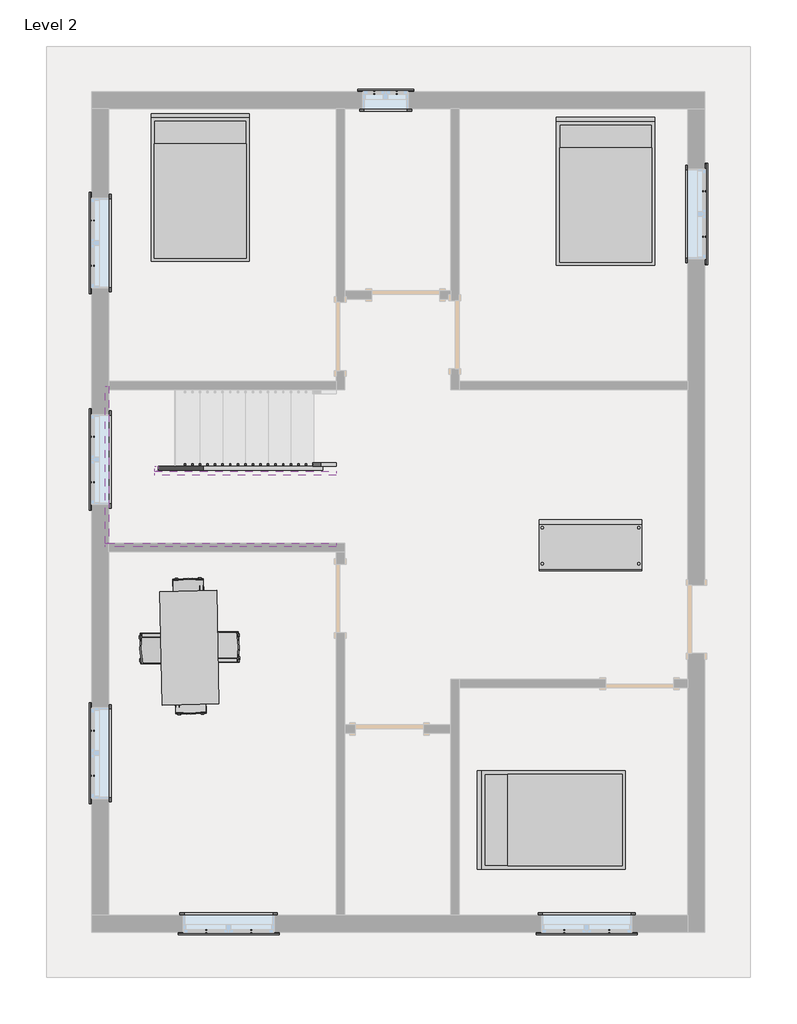
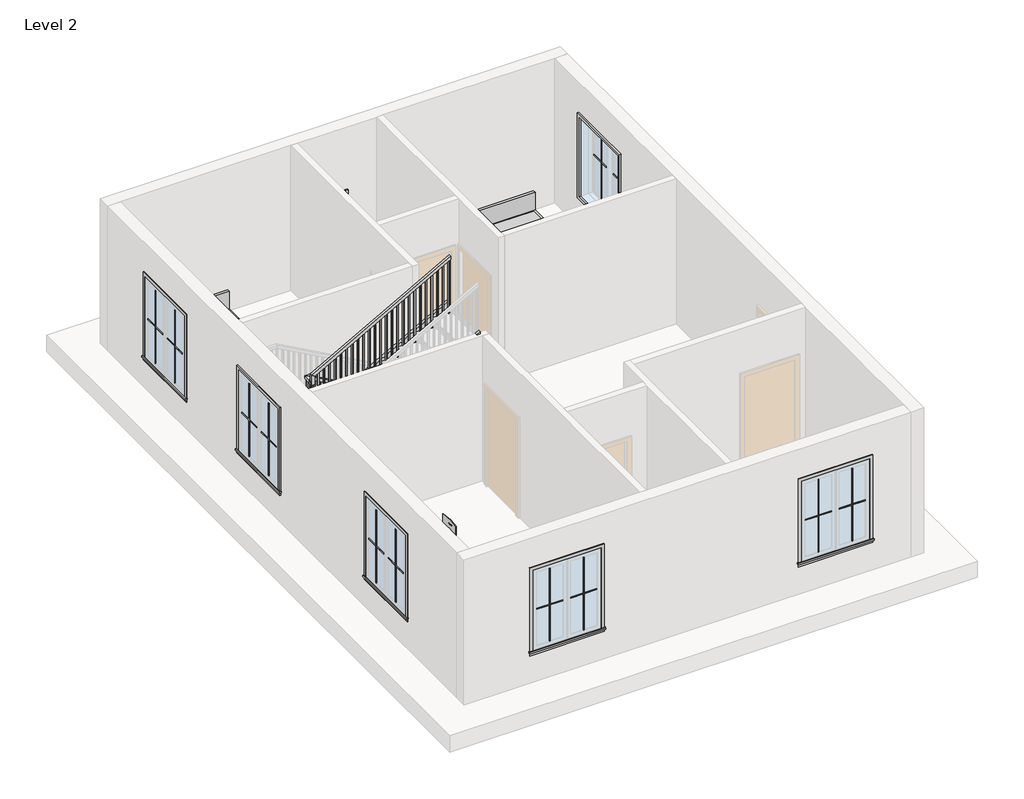
# One storey, part 2 of 2: 29 proxies, 6 members, 4 furniture elements, 1 railing.
"""IFC4 building model written with IfcOpenShell, lengths in millimetres."""

from ifc_helpers import new_model, si_unit, frame, origin, place, context, project, spatial, polyline, outline, extrude, faceted_brep, transform, mapped, element, save
from components import modern_coffee_table_17989_modern_coffee_table_17989_d3a860c8, muntin_pattern_2x2_muntin_pattern_2x2_6dad3731, muntin_pattern_2x2_muntin_pattern_2x2_a30a3345, muntin_pattern_2x2_muntin_pattern_2x2_53152e2c, muntin_pattern_2x2_muntin_pattern_2x2_e8f3e573, trim_window_exterior_flat_with_sill_92b9b949, trim_window_exterior_flat_with_sill_a665a915, trim_window_interior_flat_picture_frame_3bb882cf, trim_window_interior_flat_picture_frame_d485c387, bed_17739_bed_17739_15c61121, dining_table_w_chairs_11374_0cdfc61b

model = new_model("IFC4")

# Units and contexts
model_context = context("Model", 3, world=origin())
ifc_project = project(units=[si_unit("LENGTHUNIT", "METRE", prefix="MILLI")], contexts=[model_context])

# Site, building, storey
site = spatial("IfcSite", under=ifc_project)
building = spatial("IfcBuilding", under=site)
storey = spatial("IfcBuildingStorey", under=building, Name="Level 2", Elevation=3048.0)

# Proxies
placement = place(None, origin())
modern_coffee_table_17989_modern_coffee_table_17989_shape = modern_coffee_table_17989_modern_coffee_table_17989_d3a860c8(model_context)
element("IfcBuildingElementProxy", 1, Name="Modern_Coffee_Table_17989 : Modern_Coffee_Table_17989", ObjectType="Modern_Coffee_Table_17989 : Modern_Coffee_Table_17989", at=placement, inside=storey, context=model_context, shape_type="MappedRepresentation", body=[
    mapped(modern_coffee_table_17989_modern_coffee_table_17989_shape, transform((7937.5, 8234.1992646, 3048.0), x_axis=(1.0, 0.0, 0.0), y_axis=(0.0, 1.0, 0.0), z_axis=(0.0, 0.0, 1.0))),
])
muntin_pattern_2x2_muntin_pattern_2x2_shape = muntin_pattern_2x2_muntin_pattern_2x2_6dad3731(model_context)
element("IfcBuildingElementProxy", 2, Name="Muntin Pattern_2x2 : Muntin Pattern_2x2", ObjectType="Muntin Pattern_2x2 : Muntin Pattern_2x2", at=placement, inside=storey, context=model_context, shape_type="MappedRepresentation", body=[
    mapped(muntin_pattern_2x2_muntin_pattern_2x2_shape, transform((7961.3125, 2701.925, 4032.25), x_axis=(-1.0, 0.0, 0.0), y_axis=(0.0, -1.0, 0.0), z_axis=(0.0, 0.0, 1.0))),
])
element("IfcBuildingElementProxy", 3, Name="Muntin Pattern_2x2 : Muntin Pattern_2x2", ObjectType="Muntin Pattern_2x2 : Muntin Pattern_2x2", at=placement, inside=storey, context=model_context, shape_type="MappedRepresentation", body=[
    mapped(muntin_pattern_2x2_muntin_pattern_2x2_shape, transform((3154.3625, 2701.925, 4032.25), x_axis=(-1.0, 0.0, 0.0), y_axis=(0.0, -1.0, 0.0), z_axis=(0.0, 0.0, 1.0))),
])
element("IfcBuildingElementProxy", 4, Name="Muntin Pattern_2x2 : Muntin Pattern_2x2", ObjectType="Muntin Pattern_2x2 : Muntin Pattern_2x2", at=placement, inside=storey, context=model_context, shape_type="MappedRepresentation", body=[
    mapped(muntin_pattern_2x2_muntin_pattern_2x2_shape, transform((1025.525, 4789.4875, 4032.25), x_axis=(0.0, 1.0, 0.0), y_axis=(-1.0, 0.0, 0.0), z_axis=(0.0, 0.0, 1.0))),
])
element("IfcBuildingElementProxy", 5, Name="Muntin Pattern_2x2 : Muntin Pattern_2x2", ObjectType="Muntin Pattern_2x2 : Muntin Pattern_2x2", at=placement, inside=storey, context=model_context, shape_type="MappedRepresentation", body=[
    mapped(muntin_pattern_2x2_muntin_pattern_2x2_shape, transform((1025.525, 8732.8375, 4032.25), x_axis=(0.0, 1.0, 0.0), y_axis=(-1.0, 0.0, 0.0), z_axis=(0.0, 0.0, 1.0))),
])
element("IfcBuildingElementProxy", 6, Name="Muntin Pattern_2x2 : Muntin Pattern_2x2", ObjectType="Muntin Pattern_2x2 : Muntin Pattern_2x2", at=placement, inside=storey, context=model_context, shape_type="MappedRepresentation", body=[
    mapped(muntin_pattern_2x2_muntin_pattern_2x2_shape, transform((1025.525, 11637.9625, 4032.25), x_axis=(0.0, 1.0, 0.0), y_axis=(-1.0, 0.0, 0.0), z_axis=(0.0, 0.0, 1.0))),
])
element("IfcBuildingElementProxy", 7, Name="Muntin Pattern_2x2 : Muntin Pattern_2x2", ObjectType="Muntin Pattern_2x2 : Muntin Pattern_2x2", at=placement, inside=storey, context=model_context, shape_type="MappedRepresentation", body=[
    mapped(muntin_pattern_2x2_muntin_pattern_2x2_shape, transform((9236.075, 12634.9125, 4032.25), x_axis=(0.0, -1.0, 0.0), y_axis=(1.0, 0.0, 0.0), z_axis=(0.0, 0.0, 1.0))),
])
muntin_pattern_2x2_muntin_pattern_2x2_2_shape = muntin_pattern_2x2_muntin_pattern_2x2_a30a3345(model_context)
element("IfcBuildingElementProxy", 8, Name="Muntin Pattern_2x2 : Muntin Pattern_2x2", ObjectType="Muntin Pattern_2x2 : Muntin Pattern_2x2", at=placement, inside=storey, context=model_context, shape_type="MappedRepresentation", body=[
    mapped(muntin_pattern_2x2_muntin_pattern_2x2_2_shape, transform((7354.8875, 2701.925, 4032.25), x_axis=(1.0, 0.0, 0.0), y_axis=(0.0, 1.0, 0.0), z_axis=(0.0, 0.0, 1.0))),
])
element("IfcBuildingElementProxy", 9, Name="Muntin Pattern_2x2 : Muntin Pattern_2x2", ObjectType="Muntin Pattern_2x2 : Muntin Pattern_2x2", at=placement, inside=storey, context=model_context, shape_type="MappedRepresentation", body=[
    mapped(muntin_pattern_2x2_muntin_pattern_2x2_2_shape, transform((2547.9375, 2701.925, 4032.25), x_axis=(1.0, 0.0, 0.0), y_axis=(0.0, 1.0, 0.0), z_axis=(0.0, 0.0, 1.0))),
])
element("IfcBuildingElementProxy", 10, Name="Muntin Pattern_2x2 : Muntin Pattern_2x2", ObjectType="Muntin Pattern_2x2 : Muntin Pattern_2x2", at=placement, inside=storey, context=model_context, shape_type="MappedRepresentation", body=[
    mapped(muntin_pattern_2x2_muntin_pattern_2x2_2_shape, transform((1025.525, 5395.9125, 4032.25), x_axis=(0.0, -1.0, 0.0), y_axis=(1.0, 0.0, 0.0), z_axis=(0.0, 0.0, 1.0))),
])
element("IfcBuildingElementProxy", 11, Name="Muntin Pattern_2x2 : Muntin Pattern_2x2", ObjectType="Muntin Pattern_2x2 : Muntin Pattern_2x2", at=placement, inside=storey, context=model_context, shape_type="MappedRepresentation", body=[
    mapped(muntin_pattern_2x2_muntin_pattern_2x2_2_shape, transform((1025.525, 9339.2625, 4032.25), x_axis=(0.0, -1.0, 0.0), y_axis=(1.0, 0.0, 0.0), z_axis=(0.0, 0.0, 1.0))),
])
element("IfcBuildingElementProxy", 12, Name="Muntin Pattern_2x2 : Muntin Pattern_2x2", ObjectType="Muntin Pattern_2x2 : Muntin Pattern_2x2", at=placement, inside=storey, context=model_context, shape_type="MappedRepresentation", body=[
    mapped(muntin_pattern_2x2_muntin_pattern_2x2_2_shape, transform((1025.525, 12244.3875, 4032.25), x_axis=(0.0, -1.0, 0.0), y_axis=(1.0, 0.0, 0.0), z_axis=(0.0, 0.0, 1.0))),
])
element("IfcBuildingElementProxy", 13, Name="Muntin Pattern_2x2 : Muntin Pattern_2x2", ObjectType="Muntin Pattern_2x2 : Muntin Pattern_2x2", at=placement, inside=storey, context=model_context, shape_type="MappedRepresentation", body=[
    mapped(muntin_pattern_2x2_muntin_pattern_2x2_2_shape, transform((9236.075, 12028.4875, 4032.25), x_axis=(0.0, 1.0, 0.0), y_axis=(-1.0, 0.0, 0.0), z_axis=(0.0, 0.0, 1.0))),
])
muntin_pattern_2x2_muntin_pattern_2x2_3_shape = muntin_pattern_2x2_muntin_pattern_2x2_53152e2c(model_context)
element("IfcBuildingElementProxy", 14, Name="Muntin Pattern_2x2 : Muntin Pattern_2x2", ObjectType="Muntin Pattern_2x2 : Muntin Pattern_2x2", at=placement, inside=storey, context=model_context, shape_type="MappedRepresentation", body=[
    mapped(muntin_pattern_2x2_muntin_pattern_2x2_3_shape, transform((4808.5375, 13960.475, 4032.25), x_axis=(1.0, 0.0, 0.0), y_axis=(0.0, 1.0, 0.0), z_axis=(0.0, 0.0, 1.0))),
])
muntin_pattern_2x2_muntin_pattern_2x2_4_shape = muntin_pattern_2x2_muntin_pattern_2x2_e8f3e573(model_context)
element("IfcBuildingElementProxy", 15, Name="Muntin Pattern_2x2 : Muntin Pattern_2x2", ObjectType="Muntin Pattern_2x2 : Muntin Pattern_2x2", at=placement, inside=storey, context=model_context, shape_type="MappedRepresentation", body=[
    mapped(muntin_pattern_2x2_muntin_pattern_2x2_4_shape, transform((5110.1625, 13960.475, 4032.25), x_axis=(-1.0, 0.0, 0.0), y_axis=(0.0, -1.0, 0.0), z_axis=(0.0, 0.0, 1.0))),
])
trim_window_exterior_flat_with_sill_shape = trim_window_exterior_flat_with_sill_92b9b949(model_context)
element("IfcBuildingElementProxy", 16, Name="Trim-Window-Exterior-Flat : with Sill", ObjectType="Trim-Window-Exterior-Flat : with Sill", at=placement, inside=storey, context=model_context, shape_type="MappedRepresentation", body=[
    mapped(trim_window_exterior_flat_with_sill_shape, transform((7658.1, 2692.4, 5486.4), x_axis=(1.0, 0.0, 0.0), y_axis=(0.0, 0.0, 1.0), z_axis=(0.0, -1.0, 0.0))),
])
element("IfcBuildingElementProxy", 17, Name="Trim-Window-Exterior-Flat : with Sill", ObjectType="Trim-Window-Exterior-Flat : with Sill", at=placement, inside=storey, context=model_context, shape_type="MappedRepresentation", body=[
    mapped(trim_window_exterior_flat_with_sill_shape, transform((2851.15, 2692.4, 5486.4), x_axis=(1.0, 0.0, 0.0), y_axis=(0.0, 0.0, 1.0), z_axis=(0.0, -1.0, 0.0))),
])
element("IfcBuildingElementProxy", 18, Name="Trim-Window-Exterior-Flat : with Sill", ObjectType="Trim-Window-Exterior-Flat : with Sill", at=placement, inside=storey, context=model_context, shape_type="MappedRepresentation", body=[
    mapped(trim_window_exterior_flat_with_sill_shape, transform((1016.0, 5092.7, 5486.4), x_axis=(0.0, -1.0, 0.0), y_axis=(0.0, 0.0, 1.0), z_axis=(-1.0, 0.0, 0.0))),
])
element("IfcBuildingElementProxy", 19, Name="Trim-Window-Exterior-Flat : with Sill", ObjectType="Trim-Window-Exterior-Flat : with Sill", at=placement, inside=storey, context=model_context, shape_type="MappedRepresentation", body=[
    mapped(trim_window_exterior_flat_with_sill_shape, transform((1016.0, 9036.05, 5486.4), x_axis=(0.0, -1.0, 0.0), y_axis=(0.0, 0.0, 1.0), z_axis=(-1.0, 0.0, 0.0))),
])
element("IfcBuildingElementProxy", 20, Name="Trim-Window-Exterior-Flat : with Sill", ObjectType="Trim-Window-Exterior-Flat : with Sill", at=placement, inside=storey, context=model_context, shape_type="MappedRepresentation", body=[
    mapped(trim_window_exterior_flat_with_sill_shape, transform((1016.0, 11941.175, 5486.4), x_axis=(0.0, -1.0, 0.0), y_axis=(0.0, 0.0, 1.0), z_axis=(-1.0, 0.0, 0.0))),
])
element("IfcBuildingElementProxy", 21, Name="Trim-Window-Exterior-Flat : with Sill", ObjectType="Trim-Window-Exterior-Flat : with Sill", at=placement, inside=storey, context=model_context, shape_type="MappedRepresentation", body=[
    mapped(trim_window_exterior_flat_with_sill_shape, transform((9245.6, 12331.7, 5486.4), x_axis=(0.0, 1.0, 0.0), y_axis=(0.0, 0.0, 1.0), z_axis=(1.0, 0.0, 0.0))),
])
trim_window_exterior_flat_with_sill_2_shape = trim_window_exterior_flat_with_sill_a665a915(model_context)
element("IfcBuildingElementProxy", 22, Name="Trim-Window-Exterior-Flat : with Sill", ObjectType="Trim-Window-Exterior-Flat : with Sill", at=placement, inside=storey, context=model_context, shape_type="MappedRepresentation", body=[
    mapped(trim_window_exterior_flat_with_sill_2_shape, transform((4959.35, 13970.0, 4876.8), x_axis=(-1.0, 0.0, 0.0), y_axis=(0.0, 0.0, 1.0), z_axis=(0.0, 1.0, 0.0))),
])
trim_window_interior_flat_picture_frame_shape = trim_window_interior_flat_picture_frame_3bb882cf(model_context)
element("IfcBuildingElementProxy", 23, Name="Trim-Window-Interior-Flat : Picture Frame", ObjectType="Trim-Window-Interior-Flat : Picture Frame", at=placement, inside=storey, context=model_context, shape_type="MappedRepresentation", body=[
    mapped(trim_window_interior_flat_picture_frame_shape, transform((7658.1, 2921.0, 5486.4), x_axis=(-1.0, 0.0, 0.0), y_axis=(0.0, 0.0, 1.0), z_axis=(0.0, 1.0, 0.0))),
])
element("IfcBuildingElementProxy", 24, Name="Trim-Window-Interior-Flat : Picture Frame", ObjectType="Trim-Window-Interior-Flat : Picture Frame", at=placement, inside=storey, context=model_context, shape_type="MappedRepresentation", body=[
    mapped(trim_window_interior_flat_picture_frame_shape, transform((2851.15, 2921.0, 5486.4), x_axis=(-1.0, 0.0, 0.0), y_axis=(0.0, 0.0, 1.0), z_axis=(0.0, 1.0, 0.0))),
])
element("IfcBuildingElementProxy", 25, Name="Trim-Window-Interior-Flat : Picture Frame", ObjectType="Trim-Window-Interior-Flat : Picture Frame", at=placement, inside=storey, context=model_context, shape_type="MappedRepresentation", body=[
    mapped(trim_window_interior_flat_picture_frame_shape, transform((1244.6, 5092.7, 5486.4), x_axis=(0.0, 1.0, 0.0), y_axis=(0.0, 0.0, 1.0), z_axis=(1.0, 0.0, 0.0))),
])
element("IfcBuildingElementProxy", 26, Name="Trim-Window-Interior-Flat : Picture Frame", ObjectType="Trim-Window-Interior-Flat : Picture Frame", at=placement, inside=storey, context=model_context, shape_type="MappedRepresentation", body=[
    mapped(trim_window_interior_flat_picture_frame_shape, transform((1244.6, 9036.05, 5486.4), x_axis=(0.0, 1.0, 0.0), y_axis=(0.0, 0.0, 1.0), z_axis=(1.0, 0.0, 0.0))),
])
element("IfcBuildingElementProxy", 27, Name="Trim-Window-Interior-Flat : Picture Frame", ObjectType="Trim-Window-Interior-Flat : Picture Frame", at=placement, inside=storey, context=model_context, shape_type="MappedRepresentation", body=[
    mapped(trim_window_interior_flat_picture_frame_shape, transform((1244.6, 11941.175, 5486.4), x_axis=(0.0, 1.0, 0.0), y_axis=(0.0, 0.0, 1.0), z_axis=(1.0, 0.0, 0.0))),
])
element("IfcBuildingElementProxy", 28, Name="Trim-Window-Interior-Flat : Picture Frame", ObjectType="Trim-Window-Interior-Flat : Picture Frame", at=placement, inside=storey, context=model_context, shape_type="MappedRepresentation", body=[
    mapped(trim_window_interior_flat_picture_frame_shape, transform((9017.0, 12331.7, 5486.4), x_axis=(0.0, -1.0, 0.0), y_axis=(0.0, 0.0, 1.0), z_axis=(-1.0, 0.0, 0.0))),
])
trim_window_interior_flat_picture_frame_2_shape = trim_window_interior_flat_picture_frame_d485c387(model_context)
element("IfcBuildingElementProxy", 29, Name="Trim-Window-Interior-Flat : Picture Frame", ObjectType="Trim-Window-Interior-Flat : Picture Frame", at=placement, inside=storey, context=model_context, shape_type="MappedRepresentation", body=[
    mapped(trim_window_interior_flat_picture_frame_2_shape, transform((4959.35, 13741.4, 4876.8), x_axis=(1.0, 0.0, 0.0), y_axis=(0.0, 0.0, 1.0), z_axis=(0.0, -1.0, 0.0))),
])

# Furniture
bed_17739_bed_17739_shape = bed_17739_bed_17739_15c61121(model_context)
element("IfcFurniture", 30, ObjectType="Bed_17739 : Bed_17739", at=placement, inside=storey, context=model_context, shape_type="MappedRepresentation", body=[
    mapped(bed_17739_bed_17739_shape, transform((2470.15, 12661.9, 3048.0), x_axis=(1.0, 0.0, 0.0), y_axis=(0.0, 1.0, 0.0), z_axis=(0.0, 0.0, 1.0))),
])
element("IfcFurniture", 31, ObjectType="Bed_17739 : Bed_17739", at=placement, inside=storey, context=model_context, shape_type="MappedRepresentation", body=[
    mapped(bed_17739_bed_17739_shape, transform((7912.1, 12611.1, 3048.0), x_axis=(1.0, 0.0, 0.0), y_axis=(0.0, 1.0, 0.0), z_axis=(0.0, 0.0, 1.0))),
])
element("IfcFurniture", 32, ObjectType="Bed_17739 : Bed_17739", at=placement, inside=storey, context=model_context, shape_type="MappedRepresentation", body=[
    mapped(bed_17739_bed_17739_shape, transform((7207.25, 4197.35, 3048.0), x_axis=(0.0, 1.0, 0.0), y_axis=(-1.0, 0.0, 0.0), z_axis=(0.0, 0.0, 1.0))),
])
dining_table_w_chairs_11374_shape = dining_table_w_chairs_11374_0cdfc61b(model_context)
element("IfcFurniture", 33, ObjectType="Dining_Table_w_Chairs_11374", at=placement, inside=storey, context=model_context, shape_type="MappedRepresentation", body=[
    mapped(dining_table_w_chairs_11374_shape, transform((2420.6366388, 6492.5326572, 3048.0), x_axis=(-0.019560245774115807, 0.9998086800909743, 0.0), y_axis=(-0.9998086800909743, -0.019560245774115807, 0.0), z_axis=(0.0, 0.0, 1.0))),
])

# Members
element("IfcMember", 34, ObjectType="Stringer - 2\" Width", at=placement, inside=storey, context=model_context, shape_type="SweptSolid", body=[
    extrude(outline(polyline([(3048.0, 4295.1355783), (3255.5983948, 4295.1355783), (4582.0428392, 1907.5355783), (4233.3641651, 1907.5355783), (3048.0, 4041.1910755), (3048.0, 4295.1355783)])), frame((0.0, 8893.8068332, 0.0), z_axis=(0.0, 1.0, 0.0), x_axis=(0.0, 0.0, 1.0)), (0.0, 0.0, 1.0), 50.8),
])
element("IfcMember", 35, ObjectType="Stringer - 2\" Width", at=placement, inside=storey, context=model_context, shape_type="SweptSolid", body=[
    extrude(outline(polyline([(1856.7355783, 8944.6068332), (1907.5355783, 8944.6068332), (1907.5355783, 8877.3), (1856.7355783, 8877.3), (1856.7355783, 8944.6068332)])), frame((0.0, 0.0, 4343.4), z_axis=(0.0, 0.0, 1.0), x_axis=(1.0, 0.0, 0.0)), (0.0, 0.0, 1.0), 304.8),
])
element("IfcMember", 36, ObjectType="Stringer - 2\" Width", at=placement, inside=storey, context=model_context, shape_type="SweptSolid", body=[
    extrude(outline(polyline([(4779.5983948, 1856.7355783), (4430.9197207, 1856.7355783), (5785.5863873, 4295.1355783), (6134.2650614, 4295.1355783), (4779.5983948, 1856.7355783)])), frame((0.0, 8826.5, 0.0), z_axis=(0.0, 1.0, 0.0), x_axis=(0.0, 0.0, 1.0)), (0.0, 0.0, 1.0), 50.8),
])
element("IfcMember", 37, ObjectType="Stringer - 2\" Width", at=placement, inside=storey, context=model_context, shape_type="SweptSolid", body=[
    extrude(outline(polyline([(3048.0, 4295.1355783), (3255.5983948, 4295.1355783), (4648.2, 1788.4526889), (4648.2, 1244.6), (4601.6617086, 1244.6), (3048.0, 4041.1910755), (3048.0, 4295.1355783)])), frame((0.0, 9969.5, 0.0), z_axis=(0.0, 1.0, 0.0), x_axis=(0.0, 0.0, 1.0)), (0.0, 0.0, 1.0), 50.8),
])
element("IfcMember", 38, ObjectType="Stringer - 2\" Width", at=placement, inside=storey, context=model_context, shape_type="SweptSolid", body=[
    extrude(outline(polyline([(1193.8, 10020.3), (1244.6, 10020.3), (1244.6, 7912.1), (1193.8, 7912.1), (1193.8, 10020.3)])), frame((0.0, 0.0, 4343.4), z_axis=(0.0, 0.0, 1.0), x_axis=(1.0, 0.0, 0.0)), (0.0, 0.0, 1.0), 304.8),
])
element("IfcMember", 39, ObjectType="Stringer - 2\" Width", at=placement, inside=storey, context=model_context, shape_type="SweptSolid", body=[
    extrude(outline(polyline([(4411.3008513, 1193.8), (4343.4, 1193.8), (4343.4, 1699.2000811), (5785.5863873, 4295.1355783), (6134.2650614, 4295.1355783), (4411.3008513, 1193.8)])), frame((0.0, 7861.3, 0.0), z_axis=(0.0, 1.0, 0.0), x_axis=(0.0, 0.0, 1.0)), (0.0, 0.0, 1.0), 50.8),
])

# Railing
element("IfcRailing", 40, ObjectType="Handrail - Rectangular", at=placement, inside=storey, context=model_context, shape_type="SolidModel", body=[
    faceted_brep([(4295.1355783, 8944.6068332, 4131.7333333), (4295.1355783, 8944.6068332, 4073.620221), (4295.1355783, 8995.4068332, 4073.620221), (4295.1355783, 8995.4068332, 4131.7333333), (1932.9355783, 8944.6068332, 5444.0666667), (1882.1355783, 8944.6068332, 5414.1757765), (1882.1355783, 8995.4068332, 5414.1757765), (1932.9355783, 8995.4068332, 5444.0666667), (1932.9355783, 8944.6068332, 5486.4), (1882.1355783, 8944.6068332, 5435.6), (1882.1355783, 8995.4068332, 5435.6), (1932.9355783, 8995.4068332, 5486.4), (1856.7355783, 8944.6068332, 5486.4), (1856.7355783, 8944.6068332, 5435.6), (1805.9355783, 8995.4068332, 5435.6), (1805.9355783, 8995.4068332, 5486.4), (1856.7355783, 8868.4068332, 5486.4), (1856.7355783, 8868.4068332, 5435.6), (1805.9355783, 8868.4068332, 5435.6), (1805.9355783, 8868.4068332, 5486.4), (1856.7355783, 8826.5, 5486.4), (1805.9355783, 8826.5, 5486.4), (1805.9355783, 8775.7, 5435.6), (1856.7355783, 8775.7, 5435.6)], [[[0, 1, 2, 3]], [[1, 0, 4, 5]], [[2, 1, 5, 6]], [[3, 2, 6, 7]], [[0, 3, 7, 4]], [[5, 4, 8, 9]], [[6, 5, 9, 10]], [[7, 6, 10, 11]], [[4, 7, 11, 8]], [[9, 8, 12, 13]], [[10, 9, 13, 14]], [[11, 10, 14, 15]], [[8, 11, 15, 12]], [[13, 12, 16, 17]], [[14, 13, 17, 18]], [[15, 14, 18, 19]], [[12, 15, 19, 16]], [[20, 21, 22, 23]], [[17, 16, 20, 23]], [[18, 17, 23, 22]], [[19, 18, 22, 21]], [[16, 19, 21, 20]]]),
    faceted_brep([(1856.7355783, 8826.5, 5486.4), (1856.7355783, 8775.7, 5435.6), (1805.9355783, 8775.7, 5435.6), (1805.9355783, 8826.5, 5486.4), (1856.7355783, 8826.5, 5597.620221), (1805.9355783, 8826.5, 5627.5111111), (1805.9355783, 8775.7, 5627.5111111), (1856.7355783, 8775.7, 5597.620221)], [[[0, 1, 2, 3]], [[4, 5, 6, 7]], [[1, 0, 4, 7]], [[2, 1, 7, 6]], [[3, 2, 6, 5]], [[0, 3, 5, 4]]]),
    faceted_brep([(1805.9355783, 8826.5, 5627.5111111), (1856.7355783, 8826.5, 5597.620221), (1856.7355783, 8775.7, 5597.620221), (1805.9355783, 8775.7, 5627.5111111), (4295.1355783, 8826.5, 7010.4), (4295.1355783, 8775.7, 7010.4), (4295.1355783, 8775.7, 6952.2868876), (4295.1355783, 8826.5, 6952.2868876)], [[[0, 1, 2, 3]], [[4, 5, 6, 7]], [[1, 0, 4, 7]], [[2, 1, 7, 6]], [[3, 2, 6, 5]], [[0, 3, 5, 4]]]),
    extrude(outline(polyline([(6932.8841099, 4260.2105783), (5926.6666667, 4260.2105783), (5926.6666667, 4279.2605783), (6943.4674432, 4279.2605783), (6932.8841099, 4260.2105783)])), frame((0.0, 8791.575, 0.0), z_axis=(0.0, 1.0, 0.0), x_axis=(0.0, 0.0, 1.0)), (0.0, 0.0, 1.0), 19.05),
    extrude(outline(polyline([(6876.4396654, 4158.6105783), (5926.6666667, 4158.6105783), (5926.6666667, 4177.6605783), (6887.0229988, 4177.6605783), (6876.4396654, 4158.6105783)])), frame((0.0, 8791.575, 0.0), z_axis=(0.0, 1.0, 0.0), x_axis=(0.0, 0.0, 1.0)), (0.0, 0.0, 1.0), 19.05),
    extrude(outline(polyline([(6819.995221, 4057.0105783), (5926.6666667, 4057.0105783), (5926.6666667, 4076.0605783), (6830.5785543, 4076.0605783), (6819.995221, 4057.0105783)])), frame((0.0, 8791.575, 0.0), z_axis=(0.0, 1.0, 0.0), x_axis=(0.0, 0.0, 1.0)), (0.0, 0.0, 1.0), 19.05),
    extrude(outline(polyline([(6763.5507765, 3955.4105783), (5757.3333333, 3955.4105783), (5757.3333333, 3974.4605783), (6774.1341099, 3974.4605783), (6763.5507765, 3955.4105783)])), frame((0.0, 8791.575, 0.0), z_axis=(0.0, 1.0, 0.0), x_axis=(0.0, 0.0, 1.0)), (0.0, 0.0, 1.0), 19.05),
    extrude(outline(polyline([(6707.1063321, 3853.8105783), (5757.3333333, 3853.8105783), (5757.3333333, 3872.8605783), (6717.6896654, 3872.8605783), (6707.1063321, 3853.8105783)])), frame((0.0, 8791.575, 0.0), z_axis=(0.0, 1.0, 0.0), x_axis=(0.0, 0.0, 1.0)), (0.0, 0.0, 1.0), 19.05),
    extrude(outline(polyline([(6650.6618876, 3752.2105783), (5757.3333333, 3752.2105783), (5757.3333333, 3771.2605783), (6661.245221, 3771.2605783), (6650.6618876, 3752.2105783)])), frame((0.0, 8791.575, 0.0), z_axis=(0.0, 1.0, 0.0), x_axis=(0.0, 0.0, 1.0)), (0.0, 0.0, 1.0), 19.05),
    extrude(outline(polyline([(6594.2174432, 3650.6105783), (5588.0, 3650.6105783), (5588.0, 3669.6605783), (6604.8007765, 3669.6605783), (6594.2174432, 3650.6105783)])), frame((0.0, 8791.575, 0.0), z_axis=(0.0, 1.0, 0.0), x_axis=(0.0, 0.0, 1.0)), (0.0, 0.0, 1.0), 19.05),
    extrude(outline(polyline([(6537.7729988, 3549.0105783), (5588.0, 3549.0105783), (5588.0, 3568.0605783), (6548.3563321, 3568.0605783), (6537.7729988, 3549.0105783)])), frame((0.0, 8791.575, 0.0), z_axis=(0.0, 1.0, 0.0), x_axis=(0.0, 0.0, 1.0)), (0.0, 0.0, 1.0), 19.05),
    extrude(outline(polyline([(6481.3285543, 3447.4105783), (5588.0, 3447.4105783), (5588.0, 3466.4605783), (6491.9118876, 3466.4605783), (6481.3285543, 3447.4105783)])), frame((0.0, 8791.575, 0.0), z_axis=(0.0, 1.0, 0.0), x_axis=(0.0, 0.0, 1.0)), (0.0, 0.0, 1.0), 19.05),
    extrude(outline(polyline([(6424.8841099, 3345.8105783), (5418.6666667, 3345.8105783), (5418.6666667, 3364.8605783), (6435.4674432, 3364.8605783), (6424.8841099, 3345.8105783)])), frame((0.0, 8791.575, 0.0), z_axis=(0.0, 1.0, 0.0), x_axis=(0.0, 0.0, 1.0)), (0.0, 0.0, 1.0), 19.05),
    extrude(outline(polyline([(6368.4396654, 3244.2105783), (5418.6666667, 3244.2105783), (5418.6666667, 3263.2605783), (6379.0229988, 3263.2605783), (6368.4396654, 3244.2105783)])), frame((0.0, 8791.575, 0.0), z_axis=(0.0, 1.0, 0.0), x_axis=(0.0, 0.0, 1.0)), (0.0, 0.0, 1.0), 19.05),
    extrude(outline(polyline([(6311.995221, 3142.6105783), (5418.6666667, 3142.6105783), (5418.6666667, 3161.6605783), (6322.5785543, 3161.6605783), (6311.995221, 3142.6105783)])), frame((0.0, 8791.575, 0.0), z_axis=(0.0, 1.0, 0.0), x_axis=(0.0, 0.0, 1.0)), (0.0, 0.0, 1.0), 19.05),
    extrude(outline(polyline([(6255.5507765, 3041.0105783), (5249.3333333, 3041.0105783), (5249.3333333, 3060.0605783), (6266.1341099, 3060.0605783), (6255.5507765, 3041.0105783)])), frame((0.0, 8791.575, 0.0), z_axis=(0.0, 1.0, 0.0), x_axis=(0.0, 0.0, 1.0)), (0.0, 0.0, 1.0), 19.05),
    extrude(outline(polyline([(6199.1063321, 2939.4105783), (5249.3333333, 2939.4105783), (5249.3333333, 2958.4605783), (6209.6896654, 2958.4605783), (6199.1063321, 2939.4105783)])), frame((0.0, 8791.575, 0.0), z_axis=(0.0, 1.0, 0.0), x_axis=(0.0, 0.0, 1.0)), (0.0, 0.0, 1.0), 19.05),
    extrude(outline(polyline([(6142.6618876, 2837.8105783), (5249.3333333, 2837.8105783), (5249.3333333, 2856.8605783), (6153.245221, 2856.8605783), (6142.6618876, 2837.8105783)])), frame((0.0, 8791.575, 0.0), z_axis=(0.0, 1.0, 0.0), x_axis=(0.0, 0.0, 1.0)), (0.0, 0.0, 1.0), 19.05),
    extrude(outline(polyline([(6086.2174432, 2736.2105783), (5080.0, 2736.2105783), (5080.0, 2755.2605783), (6096.8007765, 2755.2605783), (6086.2174432, 2736.2105783)])), frame((0.0, 8791.575, 0.0), z_axis=(0.0, 1.0, 0.0), x_axis=(0.0, 0.0, 1.0)), (0.0, 0.0, 1.0), 19.05),
    extrude(outline(polyline([(6029.7729988, 2634.6105783), (5080.0, 2634.6105783), (5080.0, 2653.6605783), (6040.3563321, 2653.6605783), (6029.7729988, 2634.6105783)])), frame((0.0, 8791.575, 0.0), z_axis=(0.0, 1.0, 0.0), x_axis=(0.0, 0.0, 1.0)), (0.0, 0.0, 1.0), 19.05),
    extrude(outline(polyline([(5973.3285543, 2533.0105783), (5080.0, 2533.0105783), (5080.0, 2552.0605783), (5983.9118876, 2552.0605783), (5973.3285543, 2533.0105783)])), frame((0.0, 8791.575, 0.0), z_axis=(0.0, 1.0, 0.0), x_axis=(0.0, 0.0, 1.0)), (0.0, 0.0, 1.0), 19.05),
    extrude(outline(polyline([(5916.8841099, 2431.4105783), (4910.6666667, 2431.4105783), (4910.6666667, 2450.4605783), (5927.4674432, 2450.4605783), (5916.8841099, 2431.4105783)])), frame((0.0, 8791.575, 0.0), z_axis=(0.0, 1.0, 0.0), x_axis=(0.0, 0.0, 1.0)), (0.0, 0.0, 1.0), 19.05),
    extrude(outline(polyline([(5860.4396654, 2329.8105783), (4910.6666667, 2329.8105783), (4910.6666667, 2348.8605783), (5871.0229988, 2348.8605783), (5860.4396654, 2329.8105783)])), frame((0.0, 8791.575, 0.0), z_axis=(0.0, 1.0, 0.0), x_axis=(0.0, 0.0, 1.0)), (0.0, 0.0, 1.0), 19.05),
    extrude(outline(polyline([(5803.995221, 2228.2105783), (4910.6666667, 2228.2105783), (4910.6666667, 2247.2605783), (5814.5785543, 2247.2605783), (5803.995221, 2228.2105783)])), frame((0.0, 8791.575, 0.0), z_axis=(0.0, 1.0, 0.0), x_axis=(0.0, 0.0, 1.0)), (0.0, 0.0, 1.0), 19.05),
    extrude(outline(polyline([(5747.5507765, 2126.6105783), (4741.3333333, 2126.6105783), (4741.3333333, 2145.6605783), (5758.1341099, 2145.6605783), (5747.5507765, 2126.6105783)])), frame((0.0, 8791.575, 0.0), z_axis=(0.0, 1.0, 0.0), x_axis=(0.0, 0.0, 1.0)), (0.0, 0.0, 1.0), 19.05),
    extrude(outline(polyline([(5691.1063321, 2025.0105783), (4741.3333333, 2025.0105783), (4741.3333333, 2044.0605783), (5701.6896654, 2044.0605783), (5691.1063321, 2025.0105783)])), frame((0.0, 8791.575, 0.0), z_axis=(0.0, 1.0, 0.0), x_axis=(0.0, 0.0, 1.0)), (0.0, 0.0, 1.0), 19.05),
    extrude(outline(polyline([(5634.6618876, 1923.4105783), (4741.3333333, 1923.4105783), (4741.3333333, 1942.4605783), (5645.245221, 1942.4605783), (5634.6618876, 1923.4105783)])), frame((0.0, 8791.575, 0.0), z_axis=(0.0, 1.0, 0.0), x_axis=(0.0, 0.0, 1.0)), (0.0, 0.0, 1.0), 19.05),
    extrude(outline(polyline([(1840.8605783, 8877.9318332), (1840.8605783, 8858.8818332), (1821.8105783, 8858.8818332), (1821.8105783, 8877.9318332), (1840.8605783, 8877.9318332)])), frame((0.0, 0.0, 4572.0), z_axis=(0.0, 0.0, 1.0), x_axis=(1.0, 0.0, 0.0)), (0.0, 0.0, 1.0), 863.6),
    extrude(outline(polyline([(1866.2605783, 8960.4818332), (1847.2105783, 8960.4818332), (1847.2105783, 8979.5318332), (1866.2605783, 8979.5318332), (1866.2605783, 8960.4818332)])), frame((0.0, 0.0, 4572.0), z_axis=(0.0, 0.0, 1.0), x_axis=(1.0, 0.0, 0.0)), (0.0, 0.0, 1.0), 863.6),
    extrude(outline(polyline([(5377.1341099, 1948.8105783), (4402.6666667, 1948.8105783), (4402.6666667, 1967.8605783), (5366.5507765, 1967.8605783), (5377.1341099, 1948.8105783)])), frame((0.0, 8960.4818332, 0.0), z_axis=(0.0, 1.0, 0.0), x_axis=(0.0, 0.0, 1.0)), (0.0, 0.0, 1.0), 19.05),
    extrude(outline(polyline([(5320.6896654, 2050.4105783), (4402.6666667, 2050.4105783), (4402.6666667, 2069.4605783), (5310.1063321, 2069.4605783), (5320.6896654, 2050.4105783)])), frame((0.0, 8960.4818332, 0.0), z_axis=(0.0, 1.0, 0.0), x_axis=(0.0, 0.0, 1.0)), (0.0, 0.0, 1.0), 19.05),
    extrude(outline(polyline([(5264.245221, 2152.0105783), (4402.6666667, 2152.0105783), (4402.6666667, 2171.0605783), (5253.6618876, 2171.0605783), (5264.245221, 2152.0105783)])), frame((0.0, 8960.4818332, 0.0), z_axis=(0.0, 1.0, 0.0), x_axis=(0.0, 0.0, 1.0)), (0.0, 0.0, 1.0), 19.05),
    extrude(outline(polyline([(5207.8007765, 2253.6105783), (4233.3333333, 2253.6105783), (4233.3333333, 2272.6605783), (5197.2174432, 2272.6605783), (5207.8007765, 2253.6105783)])), frame((0.0, 8960.4818332, 0.0), z_axis=(0.0, 1.0, 0.0), x_axis=(0.0, 0.0, 1.0)), (0.0, 0.0, 1.0), 19.05),
    extrude(outline(polyline([(5151.3563321, 2355.2105783), (4233.3333333, 2355.2105783), (4233.3333333, 2374.2605783), (5140.7729988, 2374.2605783), (5151.3563321, 2355.2105783)])), frame((0.0, 8960.4818332, 0.0), z_axis=(0.0, 1.0, 0.0), x_axis=(0.0, 0.0, 1.0)), (0.0, 0.0, 1.0), 19.05),
    extrude(outline(polyline([(5094.9118876, 2456.8105783), (4233.3333333, 2456.8105783), (4233.3333333, 2475.8605783), (5084.3285543, 2475.8605783), (5094.9118876, 2456.8105783)])), frame((0.0, 8960.4818332, 0.0), z_axis=(0.0, 1.0, 0.0), x_axis=(0.0, 0.0, 1.0)), (0.0, 0.0, 1.0), 19.05),
    extrude(outline(polyline([(5038.4674432, 2558.4105783), (4064.0, 2558.4105783), (4064.0, 2577.4605783), (5027.8841099, 2577.4605783), (5038.4674432, 2558.4105783)])), frame((0.0, 8960.4818332, 0.0), z_axis=(0.0, 1.0, 0.0), x_axis=(0.0, 0.0, 1.0)), (0.0, 0.0, 1.0), 19.05),
    extrude(outline(polyline([(4982.0229988, 2660.0105783), (4064.0, 2660.0105783), (4064.0, 2679.0605783), (4971.4396654, 2679.0605783), (4982.0229988, 2660.0105783)])), frame((0.0, 8960.4818332, 0.0), z_axis=(0.0, 1.0, 0.0), x_axis=(0.0, 0.0, 1.0)), (0.0, 0.0, 1.0), 19.05),
    extrude(outline(polyline([(4925.5785543, 2761.6105783), (4064.0, 2761.6105783), (4064.0, 2780.6605783), (4914.995221, 2780.6605783), (4925.5785543, 2761.6105783)])), frame((0.0, 8960.4818332, 0.0), z_axis=(0.0, 1.0, 0.0), x_axis=(0.0, 0.0, 1.0)), (0.0, 0.0, 1.0), 19.05),
    extrude(outline(polyline([(4869.1341099, 2863.2105783), (3894.6666667, 2863.2105783), (3894.6666667, 2882.2605783), (4858.5507765, 2882.2605783), (4869.1341099, 2863.2105783)])), frame((0.0, 8960.4818332, 0.0), z_axis=(0.0, 1.0, 0.0), x_axis=(0.0, 0.0, 1.0)), (0.0, 0.0, 1.0), 19.05),
    extrude(outline(polyline([(4812.6896654, 2964.8105783), (3894.6666667, 2964.8105783), (3894.6666667, 2983.8605783), (4802.1063321, 2983.8605783), (4812.6896654, 2964.8105783)])), frame((0.0, 8960.4818332, 0.0), z_axis=(0.0, 1.0, 0.0), x_axis=(0.0, 0.0, 1.0)), (0.0, 0.0, 1.0), 19.05),
    extrude(outline(polyline([(4756.245221, 3066.4105783), (3894.6666667, 3066.4105783), (3894.6666667, 3085.4605783), (4745.6618876, 3085.4605783), (4756.245221, 3066.4105783)])), frame((0.0, 8960.4818332, 0.0), z_axis=(0.0, 1.0, 0.0), x_axis=(0.0, 0.0, 1.0)), (0.0, 0.0, 1.0), 19.05),
    extrude(outline(polyline([(4699.8007765, 3168.0105783), (3725.3333333, 3168.0105783), (3725.3333333, 3187.0605783), (4689.2174432, 3187.0605783), (4699.8007765, 3168.0105783)])), frame((0.0, 8960.4818332, 0.0), z_axis=(0.0, 1.0, 0.0), x_axis=(0.0, 0.0, 1.0)), (0.0, 0.0, 1.0), 19.05),
    extrude(outline(polyline([(4643.3563321, 3269.6105783), (3725.3333333, 3269.6105783), (3725.3333333, 3288.6605783), (4632.7729988, 3288.6605783), (4643.3563321, 3269.6105783)])), frame((0.0, 8960.4818332, 0.0), z_axis=(0.0, 1.0, 0.0), x_axis=(0.0, 0.0, 1.0)), (0.0, 0.0, 1.0), 19.05),
    extrude(outline(polyline([(4586.9118876, 3371.2105783), (3725.3333333, 3371.2105783), (3725.3333333, 3390.2605783), (4576.3285543, 3390.2605783), (4586.9118876, 3371.2105783)])), frame((0.0, 8960.4818332, 0.0), z_axis=(0.0, 1.0, 0.0), x_axis=(0.0, 0.0, 1.0)), (0.0, 0.0, 1.0), 19.05),
    extrude(outline(polyline([(4530.4674432, 3472.8105783), (3556.0, 3472.8105783), (3556.0, 3491.8605783), (4519.8841099, 3491.8605783), (4530.4674432, 3472.8105783)])), frame((0.0, 8960.4818332, 0.0), z_axis=(0.0, 1.0, 0.0), x_axis=(0.0, 0.0, 1.0)), (0.0, 0.0, 1.0), 19.05),
    extrude(outline(polyline([(4474.0229988, 3574.4105783), (3556.0, 3574.4105783), (3556.0, 3593.4605783), (4463.4396654, 3593.4605783), (4474.0229988, 3574.4105783)])), frame((0.0, 8960.4818332, 0.0), z_axis=(0.0, 1.0, 0.0), x_axis=(0.0, 0.0, 1.0)), (0.0, 0.0, 1.0), 19.05),
    extrude(outline(polyline([(4417.5785543, 3676.0105783), (3556.0, 3676.0105783), (3556.0, 3695.0605783), (4406.995221, 3695.0605783), (4417.5785543, 3676.0105783)])), frame((0.0, 8960.4818332, 0.0), z_axis=(0.0, 1.0, 0.0), x_axis=(0.0, 0.0, 1.0)), (0.0, 0.0, 1.0), 19.05),
    extrude(outline(polyline([(4361.1341099, 3777.6105783), (3386.6666667, 3777.6105783), (3386.6666667, 3796.6605783), (4350.5507765, 3796.6605783), (4361.1341099, 3777.6105783)])), frame((0.0, 8960.4818332, 0.0), z_axis=(0.0, 1.0, 0.0), x_axis=(0.0, 0.0, 1.0)), (0.0, 0.0, 1.0), 19.05),
    extrude(outline(polyline([(4304.6896654, 3879.2105783), (3386.6666667, 3879.2105783), (3386.6666667, 3898.2605783), (4294.1063321, 3898.2605783), (4304.6896654, 3879.2105783)])), frame((0.0, 8960.4818332, 0.0), z_axis=(0.0, 1.0, 0.0), x_axis=(0.0, 0.0, 1.0)), (0.0, 0.0, 1.0), 19.05),
    extrude(outline(polyline([(4248.245221, 3980.8105783), (3386.6666667, 3980.8105783), (3386.6666667, 3999.8605783), (4237.6618876, 3999.8605783), (4248.245221, 3980.8105783)])), frame((0.0, 8960.4818332, 0.0), z_axis=(0.0, 1.0, 0.0), x_axis=(0.0, 0.0, 1.0)), (0.0, 0.0, 1.0), 19.05),
    extrude(outline(polyline([(4191.8007765, 4082.4105783), (3217.3333333, 4082.4105783), (3217.3333333, 4101.4605783), (4181.2174432, 4101.4605783), (4191.8007765, 4082.4105783)])), frame((0.0, 8960.4818332, 0.0), z_axis=(0.0, 1.0, 0.0), x_axis=(0.0, 0.0, 1.0)), (0.0, 0.0, 1.0), 19.05),
    extrude(outline(polyline([(4135.3563321, 4184.0105783), (3217.3333333, 4184.0105783), (3217.3333333, 4203.0605783), (4124.7729988, 4203.0605783), (4135.3563321, 4184.0105783)])), frame((0.0, 8960.4818332, 0.0), z_axis=(0.0, 1.0, 0.0), x_axis=(0.0, 0.0, 1.0)), (0.0, 0.0, 1.0), 19.05),
    extrude(outline(polyline([(1840.8605783, 8810.625), (1840.8605783, 8791.575), (1821.8105783, 8791.575), (1821.8105783, 8810.625), (1840.8605783, 8810.625)])), frame((0.0, 0.0, 4572.0), z_axis=(0.0, 0.0, 1.0), x_axis=(1.0, 0.0, 0.0)), (0.0, 0.0, 1.0), 863.6),
    extrude(outline(polyline([(1840.8605783, 8960.4818332), (1821.8105783, 8960.4818332), (1821.8105783, 8979.5318332), (1840.8605783, 8979.5318332), (1840.8605783, 8960.4818332)])), frame((0.0, 0.0, 4572.0), z_axis=(0.0, 0.0, 1.0), x_axis=(1.0, 0.0, 0.0)), (0.0, 0.0, 1.0), 863.6),
    extrude(outline(polyline([(6941.7035543, 4276.0855783), (5926.6666667, 4276.0855783), (5926.6666667, 4295.1355783), (6952.2868876, 4295.1355783), (6941.7035543, 4276.0855783)])), frame((0.0, 8791.575, 0.0), z_axis=(0.0, 1.0, 0.0), x_axis=(0.0, 0.0, 1.0)), (0.0, 0.0, 1.0), 19.05),
    extrude(outline(polyline([(4084.2035543, 4276.0855783), (3217.3333333, 4276.0855783), (3217.3333333, 4295.1355783), (4073.620221, 4295.1355783), (4084.2035543, 4276.0855783)])), frame((0.0, 8960.4818332, 0.0), z_axis=(0.0, 1.0, 0.0), x_axis=(0.0, 0.0, 1.0)), (0.0, 0.0, 1.0), 19.05),
])

save(model, "model.ifc")

# Revit data of these elements
# Type "Modern_Coffee_Table_17989 : Modern_Coffee_Table_17989"
#   Default Elevation = 0
# Type "Muntin Pattern_2x2 : Muntin Pattern_2x2"
#   Width [instance default] = 4' - 0"
#   Thickness = 0' - 0 1/2"
#   Height [instance default] = 4' - 0"
#   Distance = 0' - 0 3/4"
#   Interior Material [instance default] = none
#   Exterior Material [instance default] = none
#   Default Elevation = 0
# Type "Trim-Window-Exterior-Flat : with Sill"
#   Trim Width = 0' - 2 1/4"
#   Trim Thickness_Picture Frame = 0' - 1 1/4"
#   Trim Thickness_with Sill = 0' - 0 3/4"
#   Sill Thickness = 0' - 1 1/4"
#   Opening Width [instance default] = 2' - 0"
#   Opening Height [instance default] = 3' - 0"
#   Default Elevation = 4' - 0"
#   Sill = yes
#   Picture Frame = no
#   Trim Material [instance default] = none
# Type "Trim-Window-Interior-Flat : Picture Frame"
#   Trim Thickness_Picture Frame = 0' - 1 1/4"
#   Trim Width = 0' - 2 1/4"
#   Trim Thickness_with Sill = 0' - 0 3/4"
#   Sill Thickness = 0' - 1 1/4"
#   Opening Width [instance default] = 2' - 0"
#   Opening Height [instance default] = 3' - 0"
#   Default Elevation = 4' - 0"
#   Sill = no
#   Picture Frame = yes
#   Trim Material [instance default] = none
# Type "Bed_17739 : Bed_17739"
#   Default Elevation = 0
# Type "Dining_Table_w_Chairs_11374"
#   Default Elevation = 0
#   Assembly Code = ""
# Type "Handrail - Rectangular"
#   Assembly Code = "C2010400"
#   built-in parameter 1008612 = 0.0416667 (stored number, unit not read)
#   built-in parameter 1008611 = 0.0416667 (stored number, unit not read)
#   built-in parameter 1008609 = 0.333333 (stored number, unit not read)
#   built-in parameter 1008604 = 0.166667 (stored number, unit not read)
#   built-in parameter 1008603 = 0.166667 (stored number, unit not read)
#   Railing Height = 3' - 0"
#   built-in parameter 1008630 = 2
#   built-in parameter 1008610 = 2
#   built-in parameter 1008618 = Baluster - Square : 3/4"
# Element 1 (IfcBuildingElementProxy, "Modern_Coffee_Table_17989 : Modern_Coffee_Table_17989")
#   Phase Created = New Construction
#   Materials on its faces: "1 Wood", "1 Glass", "1 Metal"
# Elements 2, 3, 4, 5, 6, 7, 8, 9, 10, 11, 12, 13 (IfcBuildingElementProxy, "Muntin Pattern_2x2 : Muntin Pattern_2x2")
#   Width = 1' - 6 5/8"
#   Height = 4' - 6 1/2"
#   Interior Material = Wood - Stained
#   Exterior Material = Clad - White
#   Phase Created = New Construction
#   Materials on its faces: "Clad - White", "Wood - Stained"
# Elements 14, 15 (IfcBuildingElementProxy, "Muntin Pattern_2x2 : Muntin Pattern_2x2")
#   Width = 0' - 6 5/8"
#   Height = 2' - 6 1/2"
#   Interior Material = Wood - Stained
#   Exterior Material = Clad - White
#   Phase Created = New Construction
#   Materials on its faces: "Clad - White", "Wood - Stained"
# Elements 16, 17, 18, 19, 20, 21 (IfcBuildingElementProxy, "Trim-Window-Exterior-Flat : with Sill")
#   Opening Width = 4' - 0"
#   Opening Height = 5' - 0"
#   Trim Material = Clad - White
#   Phase Created = New Construction
#   Materials on its faces: "Clad - White"
# Element 22 (IfcBuildingElementProxy, "Trim-Window-Exterior-Flat : with Sill")
#   Opening Width = 2' - 0"
#   Opening Height = 3' - 0"
#   Trim Material = Clad - White
#   Phase Created = New Construction
#   Materials on its faces: "Clad - White"
# Elements 23, 24, 25, 26, 27, 28 (IfcBuildingElementProxy, "Trim-Window-Interior-Flat : Picture Frame")
#   Opening Width = 4' - 0"
#   Opening Height = 5' - 0"
#   Trim Material = Wood - Stained
#   Phase Created = New Construction
#   Materials on its faces: "Wood - Stained"
# Element 29 (IfcBuildingElementProxy, "Trim-Window-Interior-Flat : Picture Frame")
#   Opening Width = 2' - 0"
#   Opening Height = 3' - 0"
#   Trim Material = Wood - Stained
#   Phase Created = New Construction
#   Materials on its faces: "Wood - Stained"
# Elements 30, 31, 32 (IfcFurniture, "Bed_17739 : Bed_17739")
#   Phase Created = New Construction
#   Materials on its faces: "legs", "sheets", "bed frame", "Blanket"
# Element 33 (IfcFurniture, "Dining_Table_w_Chairs_11374")
#   Phase Created = New Construction
# Elements 34, 35, 36, 37, 38, 39 (IfcMember, "Stringer - 2\" Width")
#   Phase Created = New Construction
# Element 40 (IfcRailing, "Handrail - Rectangular")
#   Phase Created = New Construction
# Materials
#   "1 Wood": class "Glass", colour RGB 81 52 39, transparency 0, Cost = 0
#   "1 Glass": class "Glass", colour RGB 236 240 239, transparency 0.85, Cost = 0
#   "1 Metal": class "Glass", colour RGB 244 244 244, transparency 0, Cost = 0
#   "Clad - White": class "Wood", colour RGB 242 242 238, transparency 0, Cost = 0
#   "Wood - Stained": class "Wood", colour RGB 224 178 126, transparency 0, Cost = 0
#   "legs": colour RGB 90 73 37, transparency 0, Cost = 0
#   "sheets": colour RGB 200 195 176, transparency 0, Cost = 0
#   "bed frame": colour RGB 90 73 37, transparency 0, Cost = 0
#   "Blanket": class "System", colour RGB 59 0 1, transparency 0, Cost = 0
